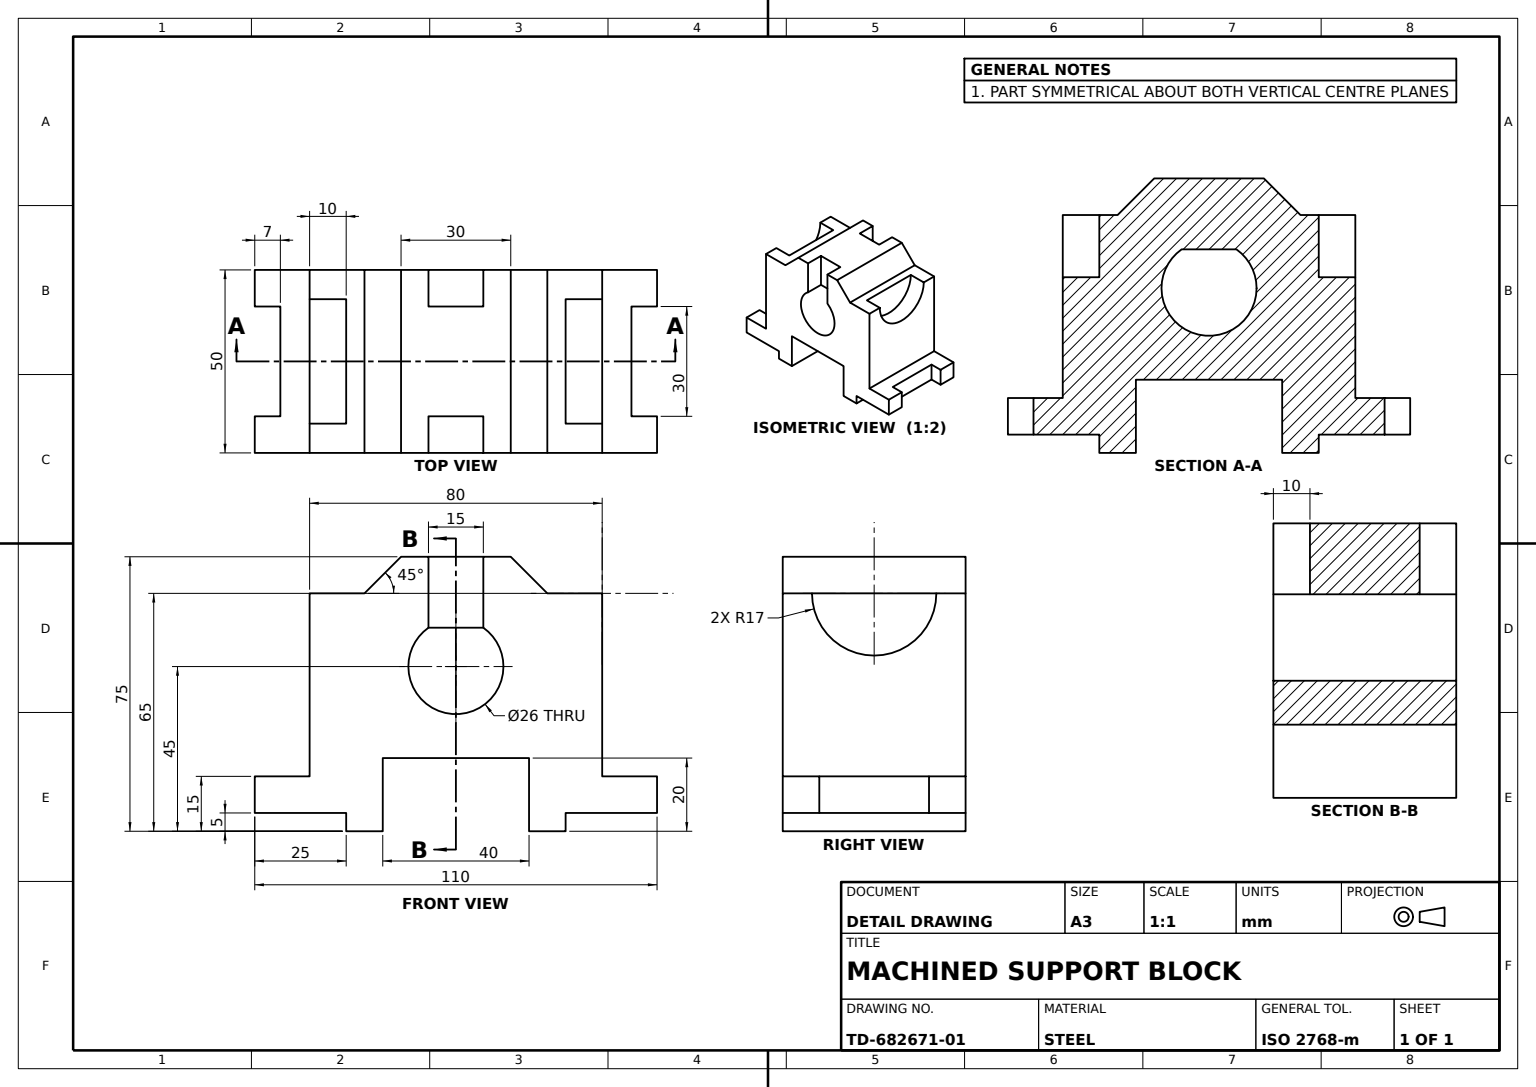
from build123d import *

# Parameters (mm, degrees)
STEPPED_BLOCK_BODY_50MM_DEPTH = 25
END_SLOT_PROFILE_30MM_W       = 30
END_SLOT_PROFILE_30MM_H       = 10
END_SLOT_CUT_7_DEEP_DEPTH     = 7
HALF_BORE_CUT_10_DEEP_DEPTH   = 10
CENTRE_BOSS_PROFILE_W         = 15
CENTRE_BOSS_PROFILE_H         = 19.381619709
CENTRE_BOSS_30MM_DEPTH        = 15


with BuildPart() as part:
    # Stepped Block Profile → Stepped Block Body 50mm (new, symmetric)
    with BuildSketch(Plane(origin=(0, 0, 0), x_dir=(0, 0, -1), z_dir=(1, 0, 0))):
        with BuildLine():
            Line((-20, -25), (20, -25))
            Line((20, -25), (20, -45))
            Line((20, -45), (30, -45))
            Line((30, -45), (30, -40))
            Line((30, -40), (55, -40))
            Line((55, -40), (55, -30))
            Line((55, -30), (40, -30))
            Line((40, -30), (40, 20))
            Line((40, 20), (25, 20))
            Line((25, 20), (15, 30))
            Line((15, 30), (7.5, 30))
            Line((7.5, 30), (7.5, 10.618380291))
            ThreePointArc((7.5, 10.618380291), (0, -13), (-7.5, 10.618380291))
            Line((-7.5, 10.618380291), (-7.5, 30))
            Line((-7.5, 30), (-15, 30))
            Line((-15, 30), (-25, 20))
            Line((-25, 20), (-40, 20))
            Line((-40, 20), (-40, -30))
            Line((-40, -30), (-55, -30))
            Line((-55, -30), (-55, -40))
            Line((-55, -40), (-30, -40))
            Line((-30, -40), (-30, -45))
            Line((-30, -45), (-20, -45))
            Line((-20, -45), (-20, -25))
        make_face()
    extrude(amount=STEPPED_BLOCK_BODY_50MM_DEPTH, both=True)

    # End Slot Profile 30mm → End Slot Cut 7 Deep (cut)
    with BuildSketch(Plane.XY.offset(55)):
        with Locations((0, -35)):
            Rectangle(END_SLOT_PROFILE_30MM_W, END_SLOT_PROFILE_30MM_H)
    end_slot_cut_7_deep = extrude(amount=-END_SLOT_CUT_7_DEEP_DEPTH, mode=Mode.SUBTRACT)

    # Half Bore Profile → Half Bore Cut 10 Deep (cut)
    with BuildSketch(Plane.XY.offset(40)):
        with BuildLine():
            Line((-17, 20), (17, 20))
            ThreePointArc((17, 20), (0, 3), (-17, 20))
        make_face()
    half_bore_cut_10_deep = extrude(amount=-HALF_BORE_CUT_10_DEEP_DEPTH, mode=Mode.SUBTRACT)

    # End Slot and Bore Mirror: End Slot Cut 7 Deep, Half Bore Cut 10 Deep across plane
    add(end_slot_cut_7_deep.mirror(Plane.XY), mode=Mode.SUBTRACT)
    add(half_bore_cut_10_deep.mirror(Plane.XY), mode=Mode.SUBTRACT)

    # Centre Boss Profile → Centre Boss 30mm (add, symmetric)
    with BuildSketch(Plane(origin=(0, 0, 0), x_dir=(0, 0, -1), z_dir=(1, 0, 0))):
        with Locations((0, 20.309190146)):
            Rectangle(CENTRE_BOSS_PROFILE_W, CENTRE_BOSS_PROFILE_H)
    extrude(amount=CENTRE_BOSS_30MM_DEPTH, both=True)


solid = part.part
